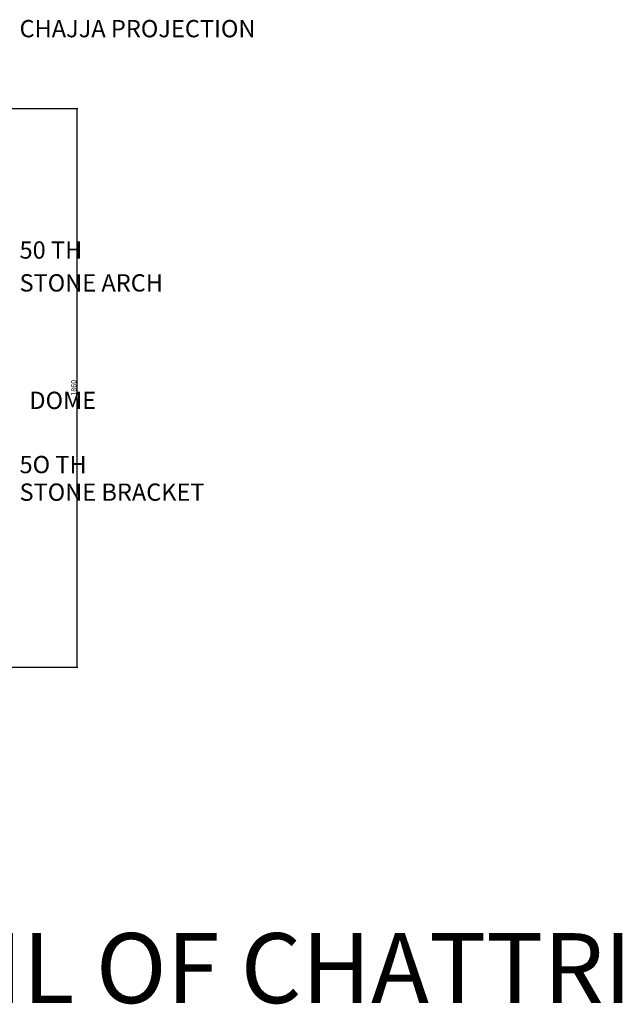
# Model space of a CAD drawing. Units: millimetres. Extents: x 498 to 8860, y -426 to 8717.
# Tile 2 of 9: x 3168 to 5174, y -426 to 2852. Entities that reach past the tile are written whole.
import ezdxf

# ---------------------------------------------------------------- set-up
doc = ezdxf.new("R2010")
doc.units = ezdxf.units.MM
doc.layers.add('A-ANNO-DIMS', color=2, linetype='Continuous', lineweight=18)
doc.layers.add('A-ANNO-TEXT', color=3, linetype='Continuous', lineweight=18)
doc.styles.get("Standard").update_dxf_attribs({"font": 'arial.ttf'})
doc.dimstyles.new('ISO-25', dxfattribs={"dimtxt": 17.5, "dimasz": 2.5, "dimexe": 1.25, "dimexo": 0.625, "dimtad": 1, "dimdec": 0, "dimtxsty": 'Standard', "dimcen": 2.5, "dimadec": 0, "dimazin": 0, "dimtfac": 1, "dimtdec": 0, "dimtmove": 0, "dimatfit": 3, "dimfxl": 1, "dimarcsym": 0})

# ---------------------------------------------------------------- blocks, each defined once
blk = doc.blocks.new('*D65')
at = {"layer": 'A-ANNO-DIMS', "color": 0, "lineweight": -2, "transparency": 16777216}
for p, q in [((2725.4, 2556.3), (3361, 2556.3)), ((3359.7, 698.8), (3359.7, 2553.8)), ((2725.4, 696.3), (3361, 696.3))]:
    blk.add_line(p, q, dxfattribs=at)
at = {"layer": 'A-ANNO-DIMS', "color": 0, "transparency": 16777216}
for points in [[(3359.3, 2553.8), (3360.1, 2553.8), (3359.7, 2556.3)], [(3359.3, 698.8), (3360.1, 698.8), (3359.7, 696.3)]]:
    blk.add_solid(points, dxfattribs=at)
at = {"layer": 'Defpoints', "color": 0, "transparency": 16777216}
for p in [(2724.7, 2556.3), (3359.7, 2556.3), (2724.7, 696.3)]:
    blk.add_point(p, dxfattribs=at)
at = {"layer": 'A-ANNO-DIMS', "color": 0, "transparency": 16777216, "insert": (3350.2, 1626.3), "char_height": 17.5, "attachment_point": 5, "rotation": 90}
blk.add_mtext('1860', dxfattribs=at)

msp = doc.modelspace()

# ---------------------------------------------------------------- texts
at = {"layer": 'A-ANNO-TEXT'}
for s, height, p in [('CHAJJA PROJECTION', 57.54038, (3167.376, 2793.519)), ('50 TH', 57.5404, (3167.376, 2056.552)), ('STONE ARCH', 57.5404, (3167.376, 1946.995)), ('DOME', 57.5404, (3200.049, 1555.834)), ('5O TH', 57.5404, (3167.376, 1342.092)), ('STONE BRACKET', 57.54038, (3167.376, 1250.22)), ('DETAIL OF CHATTRI', 232.82067, (2295.778, -422.188))]:
    msp.add_text(s, height=height, dxfattribs=at).set_placement(p)

# ---------------------------------------------------------------- dimensions: what is measured, and where the dimension line sits
at = {"layer": 'A-ANNO-DIMS'}
dim = msp.add_linear_dim(base=(3359.723, 2556.272), p1=(2724.726, 696.272), p2=(2724.726, 2556.272), angle=90, dimstyle='ISO-25', override={"dimdec": 0, "dimlfac": 1, "dimrnd": 0, "dimzin": 0, "dimdsep": 46, "dimlunit": 2}, dxfattribs=at)
dim.commit()
dim.dimension.update_dxf_attribs({"geometry": '*D65', "text_midpoint": (3350.163, 1626.272)})

doc.saveas('drawing.dxf')
